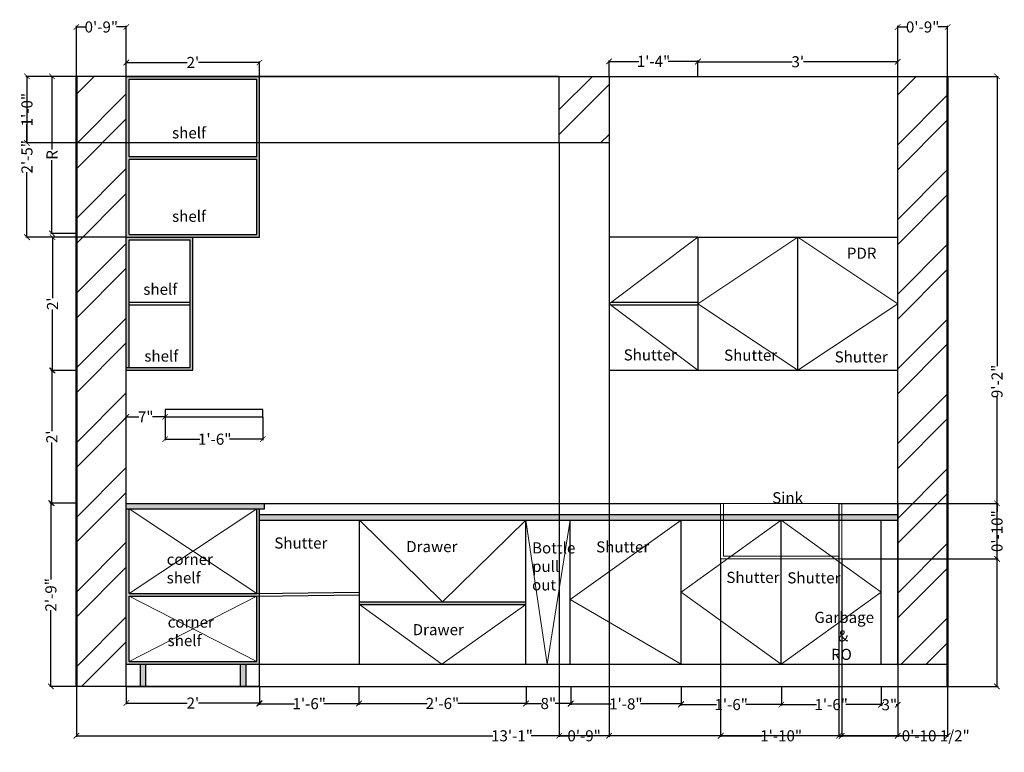
# Model space of a CAD drawing. Units: inches. Extents: x 3107 to 3291, y 1339 to 1621.
# Tile 1 of 3: x 3109 to 3286, y 1339 to 1471. Entities that reach past the tile are written whole.
import ezdxf

# ---------------------------------------------------------------- set-up
doc = ezdxf.new("R2010")
doc.units = ezdxf.units.IN
for name, color, linetype, lineweight in [('A-ANNO-DIMS', 2, 'Continuous', 18), ('A-ANNO-TEXT', 7, 'Continuous', 18), ('A-ELEV', 7, 'Continuous', 25), ('A-ELEV-OPEN', 165, 'Continuous', 13), ('A-ELEV-PATT', 8, 'Continuous', 13), ('A-FLOR-FIXT', 5, 'Continuous', 18), ('A-WALL', 7, 'Continuous', 50), ('A-WALL-PATT', 8, 'Continuous', 13)]:
    doc.layers.add(name, color=color, linetype=linetype, lineweight=lineweight)
doc.styles.get("Standard").update_dxf_attribs({"font": 'arial.ttf', "height": 2})
doc.dimstyles.get("Standard").update_dxf_attribs({"dimtxt": 2, "dimasz": 1, "dimexe": 0.18, "dimexo": 0.0625, "dimgap": 0.09, "dimtad": 0, "dimdec": 0, "dimzin": 0, "dimdsep": 46, "dimlunit": 3, "dimtxsty": 'Standard', "dimblk": 'ARCHTICK', "dimcen": 0.09, "dimadec": 0, "dimazin": 0, "dimtfac": 1, "dimtdec": 0, "dimtofl": 0, "dimtmove": 0, "dimatfit": 3, "dimfxl": 1, "dimtolj": 1, "dimtzin": 0, "dimarcsym": 0})

# ---------------------------------------------------------------- blocks, each defined once
blk = doc.blocks.new('_ArchTick')
at = {"color": 0, "linetype": 'ByBlock', "const_width": 0.15}
blk.add_lwpolyline([(-0.5, -0.5), (0.5, 0.5)], dxfattribs=at)
blk = doc.blocks.new('*D1')
at = {"layer": 'A-ANNO-DIMS', "color": 0, "lineweight": -2, "transparency": 16777216}
for p, q in [((3231.26, 1461.17), (3231.26, 1463.91)), ((3267.26, 1461.17), (3267.26, 1463.91)), ((3231.26, 1463.73), (3248.25, 1463.73)), ((3267.26, 1463.73), (3250.27, 1463.73))]:
    blk.add_line(p, q, dxfattribs=at)
at = {"layer": 'Defpoints', "color": 0, "transparency": 16777216}
for p in [(3231.26, 1463.73), (3231.26, 1461.1), (3267.26, 1461.1)]:
    blk.add_point(p, dxfattribs=at)
at = {"layer": 'A-ANNO-DIMS', "color": 0, "lineweight": -2, "transparency": 16777216, "rotation": 180}
blk.add_blockref('_ArchTick', (3231.26, 1463.73), dxfattribs=at)
at = {"layer": 'A-ANNO-DIMS', "color": 0, "lineweight": -2, "transparency": 16777216}
blk.add_blockref('_ArchTick', (3267.26, 1463.73), dxfattribs=at)
at = {"layer": 'A-ANNO-DIMS', "color": 0, "transparency": 16777216, "insert": (3249.26, 1463.73), "char_height": 2, "attachment_point": 5}
blk.add_mtext("\\A1;3'", dxfattribs=at)
blk = doc.blocks.new('*D2')
at = {"layer": 'A-ANNO-DIMS', "color": 0, "lineweight": -2, "transparency": 16777216}
for p, q in [((3215.26, 1461.17), (3215.26, 1463.98)), ((3215.26, 1463.8), (3220.61, 1463.8)), ((3231.26, 1463.8), (3225.92, 1463.8)), ((3231.26, 1461.17), (3231.26, 1463.98))]:
    blk.add_line(p, q, dxfattribs=at)
at = {"layer": 'Defpoints', "color": 0, "transparency": 16777216}
for p in [(3215.26, 1463.8), (3215.26, 1461.1), (3231.26, 1461.1)]:
    blk.add_point(p, dxfattribs=at)
at = {"layer": 'A-ANNO-DIMS', "color": 0, "lineweight": -2, "transparency": 16777216, "rotation": 180}
blk.add_blockref('_ArchTick', (3215.26, 1463.8), dxfattribs=at)
at = {"layer": 'A-ANNO-DIMS', "color": 0, "lineweight": -2, "transparency": 16777216}
blk.add_blockref('_ArchTick', (3231.26, 1463.8), dxfattribs=at)
at = {"layer": 'A-ANNO-DIMS', "color": 0, "transparency": 16777216, "insert": (3223.26, 1463.8), "char_height": 2, "attachment_point": 5}
blk.add_mtext('\\A1;1\'-4"', dxfattribs=at)
blk = doc.blocks.new('*D3')
at = {"layer": 'A-ANNO-DIMS', "color": 0, "lineweight": -2, "transparency": 16777216}
for p, q in [((3128.26, 1399.77), (3128.26, 1399.88)), ((3135.26, 1399.77), (3135.26, 1399.88)), ((3128.26, 1399.7), (3130.53, 1399.7)), ((3135.26, 1399.7), (3132.99, 1399.7))]:
    blk.add_line(p, q, dxfattribs=at)
at = {"layer": 'Defpoints', "color": 0, "transparency": 16777216}
for p in [(3128.26, 1399.7), (3128.26, 1399.7), (3135.26, 1399.7)]:
    blk.add_point(p, dxfattribs=at)
at = {"layer": 'A-ANNO-DIMS', "color": 0, "lineweight": -2, "transparency": 16777216, "rotation": 180}
blk.add_blockref('_ArchTick', (3128.26, 1399.7), dxfattribs=at)
at = {"layer": 'A-ANNO-DIMS', "color": 0, "lineweight": -2, "transparency": 16777216}
blk.add_blockref('_ArchTick', (3135.26, 1399.7), dxfattribs=at)
at = {"layer": 'A-ANNO-DIMS', "color": 0, "transparency": 16777216, "insert": (3131.76, 1399.7), "char_height": 2, "attachment_point": 5}
blk.add_mtext('\\A1;7"', dxfattribs=at)
blk = doc.blocks.new('*D4')
at = {"layer": 'A-ANNO-DIMS', "color": 0, "lineweight": -2, "transparency": 16777216}
for p, q in [((3135.26, 1399.64), (3135.26, 1395.5)), ((3152.87, 1399.64), (3152.87, 1395.5)), ((3135.26, 1395.68), (3141.53, 1395.68)), ((3152.87, 1395.68), (3146.84, 1395.68))]:
    blk.add_line(p, q, dxfattribs=at)
at = {"layer": 'Defpoints', "color": 0, "transparency": 16777216}
for p in [(3135.26, 1399.7), (3152.87, 1399.7), (3152.87, 1395.68)]:
    blk.add_point(p, dxfattribs=at)
at = {"layer": 'A-ANNO-DIMS', "color": 0, "lineweight": -2, "transparency": 16777216, "rotation": 180}
blk.add_blockref('_ArchTick', (3135.26, 1395.68), dxfattribs=at)
at = {"layer": 'A-ANNO-DIMS', "color": 0, "lineweight": -2, "transparency": 16777216}
blk.add_blockref('_ArchTick', (3152.87, 1395.68), dxfattribs=at)
at = {"layer": 'A-ANNO-DIMS', "color": 0, "transparency": 16777216, "insert": (3144.19, 1395.68), "char_height": 2, "attachment_point": 5}
blk.add_mtext('\\A1;1\'-6"', dxfattribs=at)
blk = doc.blocks.new('*D5')
at = {"layer": 'A-ANNO-DIMS', "color": 0, "lineweight": -2, "transparency": 16777216}
for p, q in [((3128.26, 1461.17), (3128.26, 1463.78)), ((3152.26, 1461.17), (3152.26, 1463.78)), ((3128.26, 1463.6), (3139.24, 1463.6)), ((3152.26, 1463.6), (3141.29, 1463.6))]:
    blk.add_line(p, q, dxfattribs=at)
at = {"layer": 'Defpoints', "color": 0, "transparency": 16777216}
for p in [(3152.26, 1463.6), (3128.26, 1461.1), (3152.26, 1461.1)]:
    blk.add_point(p, dxfattribs=at)
at = {"layer": 'A-ANNO-DIMS', "color": 0, "lineweight": -2, "transparency": 16777216, "rotation": 180}
blk.add_blockref('_ArchTick', (3128.26, 1463.6), dxfattribs=at)
at = {"layer": 'A-ANNO-DIMS', "color": 0, "lineweight": -2, "transparency": 16777216}
blk.add_blockref('_ArchTick', (3152.26, 1463.6), dxfattribs=at)
at = {"layer": 'A-ANNO-DIMS', "color": 0, "transparency": 16777216, "insert": (3140.26, 1463.6), "char_height": 2, "attachment_point": 5}
blk.add_mtext("\\A1;2'", dxfattribs=at)
blk = doc.blocks.new('*D8')
at = {"layer": 'A-ANNO-DIMS', "color": 0, "lineweight": -2, "transparency": 16777216}
for p, q in [((3119.2, 1461.1), (3114.69, 1461.1)), ((3114.87, 1461.1), (3114.87, 1447.9)), ((3114.87, 1432.76), (3114.87, 1445.96)), ((3119.2, 1432.76), (3114.69, 1432.76))]:
    blk.add_line(p, q, dxfattribs=at)
at = {"layer": 'Defpoints', "color": 0, "transparency": 16777216}
for p in [(3119.26, 1461.1), (3114.87, 1432.76), (3119.26, 1432.76)]:
    blk.add_point(p, dxfattribs=at)
at = {"layer": 'A-ANNO-DIMS', "color": 0, "lineweight": -2, "transparency": 16777216}
for p, rotation in [((3114.87, 1461.1), 90), ((3114.87, 1432.76), 270)]:
    blk.add_blockref('_ArchTick', p, dxfattribs=dict(at, rotation=rotation))
at = {"layer": 'A-ANNO-DIMS', "color": 0, "transparency": 16777216, "insert": (3114.87, 1446.93), "char_height": 2, "attachment_point": 5, "rotation": 90}
blk.add_mtext('\\A1;R', dxfattribs=at)
blk = doc.blocks.new('*D9')
at = {"layer": 'A-ANNO-DIMS', "color": 0, "lineweight": -2, "transparency": 16777216}
for p, q in [((3119.2, 1432.1), (3114.79, 1432.1)), ((3114.97, 1432.1), (3114.97, 1421.12)), ((3114.97, 1408.08), (3114.97, 1419.06)), ((3119.2, 1408.08), (3114.79, 1408.08))]:
    blk.add_line(p, q, dxfattribs=at)
at = {"layer": 'Defpoints', "color": 0, "transparency": 16777216}
for p in [(3119.26, 1432.1), (3114.97, 1408.08), (3119.26, 1408.08)]:
    blk.add_point(p, dxfattribs=at)
at = {"layer": 'A-ANNO-DIMS', "color": 0, "lineweight": -2, "transparency": 16777216}
for p, rotation in [((3114.97, 1432.1), 90), ((3114.97, 1408.08), 270)]:
    blk.add_blockref('_ArchTick', p, dxfattribs=dict(at, rotation=rotation))
at = {"layer": 'A-ANNO-DIMS', "color": 0, "transparency": 16777216, "insert": (3114.97, 1420.09), "char_height": 2, "attachment_point": 5, "rotation": 90}
blk.add_mtext("\\A1;2'", dxfattribs=at)
blk = doc.blocks.new('*D10')
at = {"layer": 'A-ANNO-DIMS', "color": 0, "lineweight": -2, "transparency": 16777216}
for p, q in [((3119.2, 1408.08), (3114.66, 1408.08)), ((3114.84, 1408.08), (3114.84, 1397.14)), ((3114.84, 1384.14), (3114.84, 1395.08)), ((3119.2, 1384.14), (3114.66, 1384.14))]:
    blk.add_line(p, q, dxfattribs=at)
at = {"layer": 'Defpoints', "color": 0, "transparency": 16777216}
for p in [(3119.26, 1408.08), (3114.84, 1384.14), (3119.26, 1384.14)]:
    blk.add_point(p, dxfattribs=at)
at = {"layer": 'A-ANNO-DIMS', "color": 0, "lineweight": -2, "transparency": 16777216}
for p, rotation in [((3114.84, 1408.08), 90), ((3114.84, 1384.14), 270)]:
    blk.add_blockref('_ArchTick', p, dxfattribs=dict(at, rotation=rotation))
at = {"layer": 'A-ANNO-DIMS', "color": 0, "transparency": 16777216, "insert": (3114.84, 1396.11), "char_height": 2, "attachment_point": 5, "rotation": 90}
blk.add_mtext("\\A1;2'", dxfattribs=at)
blk = doc.blocks.new('*D11')
at = {"layer": 'A-ANNO-DIMS', "color": 0, "lineweight": -2, "transparency": 16777216}
for p, q in [((3119.2, 1384.14), (3114.49, 1384.14)), ((3114.67, 1384.14), (3114.67, 1370.39)), ((3114.67, 1351.1), (3114.67, 1364.86)), ((3119.2, 1351.1), (3114.49, 1351.1))]:
    blk.add_line(p, q, dxfattribs=at)
at = {"layer": 'Defpoints', "color": 0, "transparency": 16777216}
for p in [(3119.26, 1384.14), (3114.67, 1351.1), (3119.26, 1351.1)]:
    blk.add_point(p, dxfattribs=at)
at = {"layer": 'A-ANNO-DIMS', "color": 0, "lineweight": -2, "transparency": 16777216}
for p, rotation in [((3114.67, 1384.14), 90), ((3114.67, 1351.1), 270)]:
    blk.add_blockref('_ArchTick', p, dxfattribs=dict(at, rotation=rotation))
at = {"layer": 'A-ANNO-DIMS', "color": 0, "transparency": 16777216, "insert": (3114.67, 1367.62), "char_height": 2, "attachment_point": 5, "rotation": 90}
blk.add_mtext('\\A1;2\'-9"', dxfattribs=at)
blk = doc.blocks.new('*D12')
at = {"layer": 'A-ANNO-DIMS', "color": 0, "lineweight": -2, "transparency": 16777216}
for p, q in [((3128.26, 1351.04), (3128.26, 1347.92)), ((3152.26, 1351.04), (3152.26, 1347.92)), ((3128.26, 1348.1), (3139.24, 1348.1)), ((3152.26, 1348.1), (3141.29, 1348.1))]:
    blk.add_line(p, q, dxfattribs=at)
at = {"layer": 'Defpoints', "color": 0, "transparency": 16777216}
for p in [(3128.26, 1351.1), (3152.26, 1351.1), (3152.26, 1348.1)]:
    blk.add_point(p, dxfattribs=at)
at = {"layer": 'A-ANNO-DIMS', "color": 0, "lineweight": -2, "transparency": 16777216, "rotation": 180}
blk.add_blockref('_ArchTick', (3128.26, 1348.1), dxfattribs=at)
at = {"layer": 'A-ANNO-DIMS', "color": 0, "lineweight": -2, "transparency": 16777216}
blk.add_blockref('_ArchTick', (3152.26, 1348.1), dxfattribs=at)
at = {"layer": 'A-ANNO-DIMS', "color": 0, "transparency": 16777216, "insert": (3140.26, 1348.1), "char_height": 2, "attachment_point": 5}
blk.add_mtext("\\A1;2'", dxfattribs=at)
blk = doc.blocks.new('*D13')
at = {"layer": 'A-ANNO-DIMS', "color": 0, "lineweight": -2, "transparency": 16777216}
for p, q in [((3152.26, 1351.04), (3152.26, 1347.81)), ((3170.18, 1351.04), (3170.18, 1347.81)), ((3152.26, 1347.99), (3158.57, 1347.99)), ((3170.18, 1347.99), (3163.87, 1347.99))]:
    blk.add_line(p, q, dxfattribs=at)
at = {"layer": 'Defpoints', "color": 0, "transparency": 16777216}
for p in [(3152.26, 1351.1), (3170.18, 1351.1), (3170.18, 1347.99)]:
    blk.add_point(p, dxfattribs=at)
at = {"layer": 'A-ANNO-DIMS', "color": 0, "lineweight": -2, "transparency": 16777216, "rotation": 180}
blk.add_blockref('_ArchTick', (3152.26, 1347.99), dxfattribs=at)
at = {"layer": 'A-ANNO-DIMS', "color": 0, "lineweight": -2, "transparency": 16777216}
blk.add_blockref('_ArchTick', (3170.18, 1347.99), dxfattribs=at)
at = {"layer": 'A-ANNO-DIMS', "color": 0, "transparency": 16777216, "insert": (3161.22, 1347.99), "char_height": 2, "attachment_point": 5}
blk.add_mtext('\\A1;1\'-6"', dxfattribs=at)
blk = doc.blocks.new('*D14')
at = {"layer": 'A-ANNO-DIMS', "color": 0, "lineweight": -2, "transparency": 16777216}
for p, q in [((3170.18, 1351.04), (3170.18, 1347.85)), ((3200.29, 1351.04), (3200.29, 1347.85)), ((3170.18, 1348.03), (3182.47, 1348.03)), ((3200.29, 1348.03), (3188, 1348.03))]:
    blk.add_line(p, q, dxfattribs=at)
at = {"layer": 'Defpoints', "color": 0, "transparency": 16777216}
for p in [(3170.18, 1351.1), (3200.29, 1351.1), (3200.29, 1348.03)]:
    blk.add_point(p, dxfattribs=at)
at = {"layer": 'A-ANNO-DIMS', "color": 0, "lineweight": -2, "transparency": 16777216, "rotation": 180}
blk.add_blockref('_ArchTick', (3170.18, 1348.03), dxfattribs=at)
at = {"layer": 'A-ANNO-DIMS', "color": 0, "lineweight": -2, "transparency": 16777216}
blk.add_blockref('_ArchTick', (3200.29, 1348.03), dxfattribs=at)
at = {"layer": 'A-ANNO-DIMS', "color": 0, "transparency": 16777216, "insert": (3185.23, 1348.03), "char_height": 2, "attachment_point": 5}
blk.add_mtext('\\A1;2\'-6"', dxfattribs=at)
blk = doc.blocks.new('*D15')
at = {"layer": 'A-ANNO-DIMS', "color": 0, "lineweight": -2, "transparency": 16777216}
for p, q in [((3200.29, 1351.04), (3200.29, 1347.84)), ((3208.34, 1351.04), (3208.34, 1347.84)), ((3200.29, 1348.02), (3203.07, 1348.02)), ((3208.34, 1348.02), (3205.55, 1348.02))]:
    blk.add_line(p, q, dxfattribs=at)
at = {"layer": 'Defpoints', "color": 0, "transparency": 16777216}
for p in [(3200.29, 1351.1), (3208.34, 1351.1), (3208.34, 1348.02)]:
    blk.add_point(p, dxfattribs=at)
at = {"layer": 'A-ANNO-DIMS', "color": 0, "lineweight": -2, "transparency": 16777216, "rotation": 180}
blk.add_blockref('_ArchTick', (3200.29, 1348.02), dxfattribs=at)
at = {"layer": 'A-ANNO-DIMS', "color": 0, "lineweight": -2, "transparency": 16777216}
blk.add_blockref('_ArchTick', (3208.34, 1348.02), dxfattribs=at)
at = {"layer": 'A-ANNO-DIMS', "color": 0, "transparency": 16777216, "insert": (3204.31, 1348.02), "char_height": 2, "attachment_point": 5}
blk.add_mtext('\\A1;8"', dxfattribs=at)
blk = doc.blocks.new('*D16')
at = {"layer": 'A-ANNO-DIMS', "color": 0, "lineweight": -2, "transparency": 16777216}
for p, q in [((3208.34, 1351.04), (3208.34, 1347.77)), ((3228.23, 1351.04), (3228.23, 1347.77)), ((3208.34, 1347.95), (3215.63, 1347.95)), ((3228.23, 1347.95), (3220.94, 1347.95))]:
    blk.add_line(p, q, dxfattribs=at)
at = {"layer": 'Defpoints', "color": 0, "transparency": 16777216}
for p in [(3208.34, 1351.1), (3228.23, 1351.1), (3228.23, 1347.95)]:
    blk.add_point(p, dxfattribs=at)
at = {"layer": 'A-ANNO-DIMS', "color": 0, "lineweight": -2, "transparency": 16777216, "rotation": 180}
blk.add_blockref('_ArchTick', (3208.34, 1347.95), dxfattribs=at)
at = {"layer": 'A-ANNO-DIMS', "color": 0, "lineweight": -2, "transparency": 16777216}
blk.add_blockref('_ArchTick', (3228.23, 1347.95), dxfattribs=at)
at = {"layer": 'A-ANNO-DIMS', "color": 0, "transparency": 16777216, "insert": (3218.28, 1347.95), "char_height": 2, "attachment_point": 5}
blk.add_mtext('\\A1;1\'-8"', dxfattribs=at)
blk = doc.blocks.new('*D17')
at = {"layer": 'A-ANNO-DIMS', "color": 0, "lineweight": -2, "transparency": 16777216}
for p, q in [((3228.23, 1351.04), (3228.23, 1347.65)), ((3246.3, 1351.04), (3246.3, 1347.65)), ((3228.23, 1347.83), (3234.61, 1347.83)), ((3246.3, 1347.83), (3239.92, 1347.83))]:
    blk.add_line(p, q, dxfattribs=at)
at = {"layer": 'Defpoints', "color": 0, "transparency": 16777216}
for p in [(3228.23, 1351.1), (3246.3, 1351.1), (3246.3, 1347.83)]:
    blk.add_point(p, dxfattribs=at)
at = {"layer": 'A-ANNO-DIMS', "color": 0, "lineweight": -2, "transparency": 16777216, "rotation": 180}
blk.add_blockref('_ArchTick', (3228.23, 1347.83), dxfattribs=at)
at = {"layer": 'A-ANNO-DIMS', "color": 0, "lineweight": -2, "transparency": 16777216}
blk.add_blockref('_ArchTick', (3246.3, 1347.83), dxfattribs=at)
at = {"layer": 'A-ANNO-DIMS', "color": 0, "transparency": 16777216, "insert": (3237.26, 1347.83), "char_height": 2, "attachment_point": 5}
blk.add_mtext('\\A1;1\'-6"', dxfattribs=at)
blk = doc.blocks.new('*D18')
at = {"layer": 'A-ANNO-DIMS', "color": 0, "lineweight": -2, "transparency": 16777216}
for p, q in [((3246.3, 1351.04), (3246.3, 1347.65)), ((3264.26, 1351.04), (3264.26, 1347.65)), ((3246.3, 1347.83), (3252.63, 1347.83)), ((3264.26, 1347.83), (3257.93, 1347.83))]:
    blk.add_line(p, q, dxfattribs=at)
at = {"layer": 'Defpoints', "color": 0, "transparency": 16777216}
for p in [(3246.3, 1351.1), (3264.26, 1351.1), (3264.26, 1347.83)]:
    blk.add_point(p, dxfattribs=at)
at = {"layer": 'A-ANNO-DIMS', "color": 0, "lineweight": -2, "transparency": 16777216, "rotation": 180}
blk.add_blockref('_ArchTick', (3246.3, 1347.83), dxfattribs=at)
at = {"layer": 'A-ANNO-DIMS', "color": 0, "lineweight": -2, "transparency": 16777216}
blk.add_blockref('_ArchTick', (3264.26, 1347.83), dxfattribs=at)
at = {"layer": 'A-ANNO-DIMS', "color": 0, "transparency": 16777216, "insert": (3255.28, 1347.83), "char_height": 2, "attachment_point": 5}
blk.add_mtext('\\A1;1\'-6"', dxfattribs=at)
blk = doc.blocks.new('*D19')
at = {"layer": 'A-ANNO-DIMS', "color": 0, "lineweight": -2, "transparency": 16777216}
for p, q in [((3264.26, 1351.04), (3264.26, 1347.62)), ((3267.26, 1351.04), (3267.26, 1347.62)), ((3264.26, 1347.8), (3264.52, 1347.8)), ((3267.26, 1347.8), (3267, 1347.8))]:
    blk.add_line(p, q, dxfattribs=at)
at = {"layer": 'Defpoints', "color": 0, "transparency": 16777216}
for p in [(3264.26, 1351.1), (3267.26, 1351.1), (3267.26, 1347.8)]:
    blk.add_point(p, dxfattribs=at)
at = {"layer": 'A-ANNO-DIMS', "color": 0, "lineweight": -2, "transparency": 16777216, "rotation": 180}
blk.add_blockref('_ArchTick', (3264.26, 1347.8), dxfattribs=at)
at = {"layer": 'A-ANNO-DIMS', "color": 0, "lineweight": -2, "transparency": 16777216}
blk.add_blockref('_ArchTick', (3267.26, 1347.8), dxfattribs=at)
at = {"layer": 'A-ANNO-DIMS', "color": 0, "transparency": 16777216, "insert": (3265.76, 1347.8), "char_height": 2, "attachment_point": 5}
blk.add_mtext('\\A1;3"', dxfattribs=at)
blk = doc.blocks.new('*D68')
at = {"layer": 'A-ANNO-DIMS', "color": 0, "lineweight": -2, "transparency": 16777216}
for p, q in [((3119.26, 1351.04), (3119.26, 1342.02)), ((3276.26, 1351.04), (3276.26, 1342.02)), ((3119.26, 1342.2), (3194.33, 1342.2)), ((3276.26, 1342.2), (3201.19, 1342.2))]:
    blk.add_line(p, q, dxfattribs=at)
at = {"layer": 'Defpoints', "color": 0, "transparency": 16777216}
for p in [(3119.26, 1351.1), (3276.26, 1351.1), (3276.26, 1342.2)]:
    blk.add_point(p, dxfattribs=at)
at = {"layer": 'A-ANNO-DIMS', "color": 0, "lineweight": -2, "transparency": 16777216, "rotation": 180}
blk.add_blockref('_ArchTick', (3119.26, 1342.2), dxfattribs=at)
at = {"layer": 'A-ANNO-DIMS', "color": 0, "lineweight": -2, "transparency": 16777216}
blk.add_blockref('_ArchTick', (3276.26, 1342.2), dxfattribs=at)
at = {"layer": 'A-ANNO-DIMS', "color": 0, "transparency": 16777216, "insert": (3197.76, 1342.2), "char_height": 2, "attachment_point": 5}
blk.add_mtext('\\A1;13\'-1"', dxfattribs=at)
blk = doc.blocks.new('*D69')
at = {"layer": 'A-ANNO-DIMS', "color": 0, "lineweight": -2, "transparency": 16777216}
for p, q in [((3276.32, 1461.1), (3285.34, 1461.1)), ((3285.16, 1461.1), (3285.16, 1408.85)), ((3285.16, 1351.1), (3285.16, 1403.36)), ((3276.32, 1351.1), (3285.34, 1351.1))]:
    blk.add_line(p, q, dxfattribs=at)
at = {"layer": 'Defpoints', "color": 0, "transparency": 16777216}
for p in [(3276.26, 1461.1), (3285.16, 1461.1), (3276.26, 1351.1)]:
    blk.add_point(p, dxfattribs=at)
at = {"layer": 'A-ANNO-DIMS', "color": 0, "lineweight": -2, "transparency": 16777216}
for p, rotation in [((3285.16, 1461.1), 90), ((3285.16, 1351.1), 270)]:
    blk.add_blockref('_ArchTick', p, dxfattribs=dict(at, rotation=rotation))
at = {"layer": 'A-ANNO-DIMS', "color": 0, "transparency": 16777216, "insert": (3285.16, 1406.1), "char_height": 2, "attachment_point": 5, "rotation": 90}
blk.add_mtext('\\A1;9\'-2"', dxfattribs=at)
blk = doc.blocks.new('*D70')
at = {"layer": 'A-ANNO-DIMS', "color": 0, "lineweight": -2, "transparency": 16777216}
for p, q in [((3128.2, 1461.1), (3110.18, 1461.1)), ((3110.36, 1461.1), (3110.36, 1449.37)), ((3110.36, 1432.1), (3110.36, 1443.84)), ((3128.2, 1432.1), (3110.18, 1432.1))]:
    blk.add_line(p, q, dxfattribs=at)
at = {"layer": 'Defpoints', "color": 0, "transparency": 16777216}
for p in [(3110.36, 1461.1), (3128.26, 1461.1), (3128.26, 1432.1)]:
    blk.add_point(p, dxfattribs=at)
at = {"layer": 'A-ANNO-DIMS', "color": 0, "lineweight": -2, "transparency": 16777216}
for p, rotation in [((3110.36, 1461.1), 90), ((3110.36, 1432.1), 270)]:
    blk.add_blockref('_ArchTick', p, dxfattribs=dict(at, rotation=rotation))
at = {"layer": 'A-ANNO-DIMS', "color": 0, "transparency": 16777216, "insert": (3110.36, 1446.6), "char_height": 2, "attachment_point": 5, "rotation": 90}
blk.add_mtext('\\A1;2\'-5"', dxfattribs=at)
blk = doc.blocks.new('*D71')
at = {"layer": 'A-ANNO-DIMS', "color": 0, "lineweight": -2, "transparency": 16777216}
for p, q in [((3119.26, 1461.17), (3119.26, 1470.18)), ((3119.26, 1470), (3121.01, 1470)), ((3128.26, 1470), (3126.51, 1470)), ((3128.26, 1461.17), (3128.26, 1470.18))]:
    blk.add_line(p, q, dxfattribs=at)
at = {"layer": 'Defpoints', "color": 0, "transparency": 16777216}
for p in [(3128.26, 1470), (3119.26, 1461.1), (3128.26, 1461.1)]:
    blk.add_point(p, dxfattribs=at)
at = {"layer": 'A-ANNO-DIMS', "color": 0, "lineweight": -2, "transparency": 16777216, "rotation": 180}
blk.add_blockref('_ArchTick', (3119.26, 1470), dxfattribs=at)
at = {"layer": 'A-ANNO-DIMS', "color": 0, "lineweight": -2, "transparency": 16777216}
blk.add_blockref('_ArchTick', (3128.26, 1470), dxfattribs=at)
at = {"layer": 'A-ANNO-DIMS', "color": 0, "transparency": 16777216, "insert": (3123.76, 1470), "char_height": 2, "attachment_point": 5}
blk.add_mtext('\\A1;0\'-9"', dxfattribs=at)
blk = doc.blocks.new('*D72')
at = {"layer": 'A-ANNO-DIMS', "color": 0, "lineweight": -2, "transparency": 16777216}
for p, q in [((3267.26, 1461.17), (3267.26, 1470.18)), ((3267.26, 1470), (3269.01, 1470)), ((3276.26, 1470), (3274.51, 1470)), ((3276.26, 1461.17), (3276.26, 1470.18))]:
    blk.add_line(p, q, dxfattribs=at)
at = {"layer": 'Defpoints', "color": 0, "transparency": 16777216}
for p in [(3276.26, 1470), (3267.26, 1461.1), (3276.26, 1461.1)]:
    blk.add_point(p, dxfattribs=at)
at = {"layer": 'A-ANNO-DIMS', "color": 0, "lineweight": -2, "transparency": 16777216, "rotation": 180}
blk.add_blockref('_ArchTick', (3267.26, 1470), dxfattribs=at)
at = {"layer": 'A-ANNO-DIMS', "color": 0, "lineweight": -2, "transparency": 16777216}
blk.add_blockref('_ArchTick', (3276.26, 1470), dxfattribs=at)
at = {"layer": 'A-ANNO-DIMS', "color": 0, "transparency": 16777216, "insert": (3271.76, 1470), "char_height": 2, "attachment_point": 5}
blk.add_mtext('\\A1;0\'-9"', dxfattribs=at)
blk = doc.blocks.new('*D73')
at = {"layer": 'A-ANNO-DIMS', "color": 0, "lineweight": -2, "transparency": 16777216}
for p, q in [((3206.2, 1461.1), (3110.18, 1461.1)), ((3110.36, 1461.1), (3110.36, 1457.76)), ((3110.36, 1449.1), (3110.36, 1452.45)), ((3206.2, 1449.1), (3110.18, 1449.1))]:
    blk.add_line(p, q, dxfattribs=at)
at = {"layer": 'Defpoints', "color": 0, "transparency": 16777216}
for p in [(3110.36, 1461.1), (3206.26, 1461.1), (3206.26, 1449.1)]:
    blk.add_point(p, dxfattribs=at)
at = {"layer": 'A-ANNO-DIMS', "color": 0, "lineweight": -2, "transparency": 16777216}
for p, rotation in [((3110.36, 1461.1), 90), ((3110.36, 1449.1), 270)]:
    blk.add_blockref('_ArchTick', p, dxfattribs=dict(at, rotation=rotation))
at = {"layer": 'A-ANNO-DIMS', "color": 0, "transparency": 16777216, "insert": (3110.36, 1455.1), "char_height": 2, "attachment_point": 5, "rotation": 90}
blk.add_mtext('\\A1;1\'-0"', dxfattribs=at)
blk = doc.blocks.new('*D74')
at = {"layer": 'A-ANNO-DIMS', "color": 0, "lineweight": -2, "transparency": 16777216}
for p, q in [((3206.26, 1449.04), (3206.26, 1342.02)), ((3215.26, 1449.04), (3215.26, 1342.02)), ((3206.26, 1342.2), (3208.01, 1342.2)), ((3215.26, 1342.2), (3213.51, 1342.2))]:
    blk.add_line(p, q, dxfattribs=at)
at = {"layer": 'Defpoints', "color": 0, "transparency": 16777216}
for p in [(3206.26, 1449.1), (3215.26, 1449.1), (3215.26, 1342.2)]:
    blk.add_point(p, dxfattribs=at)
at = {"layer": 'A-ANNO-DIMS', "color": 0, "lineweight": -2, "transparency": 16777216, "rotation": 180}
blk.add_blockref('_ArchTick', (3206.26, 1342.2), dxfattribs=at)
at = {"layer": 'A-ANNO-DIMS', "color": 0, "lineweight": -2, "transparency": 16777216}
blk.add_blockref('_ArchTick', (3215.26, 1342.2), dxfattribs=at)
at = {"layer": 'A-ANNO-DIMS', "color": 0, "transparency": 16777216, "insert": (3210.76, 1342.2), "char_height": 2, "attachment_point": 5}
blk.add_mtext('\\A1;0\'-9"', dxfattribs=at)
blk = doc.blocks.new('*D75')
at = {"layer": 'A-ANNO-DIMS', "color": 0, "lineweight": -2, "transparency": 16777216}
for p, q in [((3235.36, 1374.04), (3235.36, 1342.02)), ((3257.17, 1374.04), (3257.17, 1342.02)), ((3235.36, 1342.2), (3242.83, 1342.2)), ((3257.17, 1342.2), (3249.69, 1342.2))]:
    blk.add_line(p, q, dxfattribs=at)
at = {"layer": 'Defpoints', "color": 0, "transparency": 16777216}
for p in [(3235.36, 1374.1), (3257.17, 1374.1), (3257.17, 1342.2)]:
    blk.add_point(p, dxfattribs=at)
at = {"layer": 'A-ANNO-DIMS', "color": 0, "lineweight": -2, "transparency": 16777216, "rotation": 180}
blk.add_blockref('_ArchTick', (3235.36, 1342.2), dxfattribs=at)
at = {"layer": 'A-ANNO-DIMS', "color": 0, "lineweight": -2, "transparency": 16777216}
blk.add_blockref('_ArchTick', (3257.17, 1342.2), dxfattribs=at)
at = {"layer": 'A-ANNO-DIMS', "color": 0, "transparency": 16777216, "insert": (3246.26, 1342.2), "char_height": 2, "attachment_point": 5}
blk.add_mtext('\\A1;1\'-10"', dxfattribs=at)
blk = doc.blocks.new('*D76')
at = {"layer": 'A-ANNO-DIMS', "color": 0, "lineweight": -2, "transparency": 16777216}
for p, q in [((3256.73, 1384.1), (3285.34, 1384.1)), ((3285.16, 1384.1), (3285.16, 1382.63)), ((3285.16, 1374.1), (3285.16, 1375.58)), ((3257.23, 1374.1), (3285.34, 1374.1))]:
    blk.add_line(p, q, dxfattribs=at)
at = {"layer": 'Defpoints', "color": 0, "transparency": 16777216}
for p in [(3256.67, 1384.1), (3285.16, 1384.1), (3257.17, 1374.1)]:
    blk.add_point(p, dxfattribs=at)
at = {"layer": 'A-ANNO-DIMS', "color": 0, "lineweight": -2, "transparency": 16777216}
for p, rotation in [((3285.16, 1384.1), 90), ((3285.16, 1374.1), 270)]:
    blk.add_blockref('_ArchTick', p, dxfattribs=dict(at, rotation=rotation))
at = {"layer": 'A-ANNO-DIMS', "color": 0, "transparency": 16777216, "insert": (3285.16, 1379.1), "char_height": 2, "attachment_point": 5, "rotation": 90}
blk.add_mtext('\\A1;0\'-10"', dxfattribs=at)
blk = doc.blocks.new('*D77')
at = {"layer": 'A-ANNO-DIMS', "color": 0, "lineweight": -2, "transparency": 16777216}
for p, q in [((3256.67, 1384.04), (3256.67, 1342.02)), ((3267.26, 1384.04), (3267.26, 1342.02)), ((3256.67, 1342.2), (3267.26, 1342.2)), ((3267.26, 1342.2), (3268.26, 1342.2))]:
    blk.add_line(p, q, dxfattribs=at)
at = {"layer": 'Defpoints', "color": 0, "transparency": 16777216}
for p in [(3256.67, 1384.1), (3267.26, 1384.1), (3267.26, 1342.2)]:
    blk.add_point(p, dxfattribs=at)
at = {"layer": 'A-ANNO-DIMS', "color": 0, "lineweight": -2, "transparency": 16777216, "rotation": 180}
blk.add_blockref('_ArchTick', (3256.67, 1342.2), dxfattribs=at)
at = {"layer": 'A-ANNO-DIMS', "color": 0, "lineweight": -2, "transparency": 16777216}
blk.add_blockref('_ArchTick', (3267.26, 1342.2), dxfattribs=at)
at = {"layer": 'A-ANNO-DIMS', "color": 0, "transparency": 16777216, "insert": (3274.12, 1342.2), "char_height": 2, "attachment_point": 5}
blk.add_mtext('\\A1;0\'-10 1/2"', dxfattribs=at)

msp = doc.modelspace()

# ---------------------------------------------------------------- hatches: boundary and pattern name
at = {"layer": 'A-ELEV-PATT'}
h = msp.add_hatch(color=256, dxfattribs=at)
h.dxf.hatch_style = 1
h.paths.add_polyline_path([(3152.26, 1461.1), (3128.26, 1461.1), (3128.26, 1432.1), (3152.26, 1432.1)])
h.paths.add_polyline_path([(3151.76, 1446.6), (3128.76, 1446.6), (3128.76, 1460.6), (3151.76, 1460.6)], flags=16)
h.paths.add_polyline_path([(3151.76, 1446.1), (3151.76, 1432.6), (3128.76, 1432.6), (3128.76, 1446.1)], flags=16)
h.paths.add_polyline_path([(3140.26, 1432.1), (3128.26, 1432.1), (3128.26, 1408.6), (3128.76, 1408.6), (3128.76, 1431.6), (3139.76, 1431.6), (3139.76, 1408.6), (3128.26, 1408.6), (3128.26, 1408.1), (3140.26, 1408.1)])
h.paths.add_polyline_path([(3135.93, 1433.74), (3142.93, 1433.74), (3142.93, 1437.86), (3135.93, 1437.86)], flags=8)
h.paths.add_polyline_path([(3135.93, 1448.78), (3142.93, 1448.78), (3142.93, 1452.9), (3135.93, 1452.9)], flags=8)
h = msp.add_hatch(color=256, dxfattribs=at)
h.dxf.hatch_style = 1
h.paths.add_polyline_path([(3152.26, 1383.1), (3151.76, 1383.1), (3151.76, 1367.85), (3128.76, 1367.85), (3128.76, 1383.1), (3128.26, 1383.1), (3128.26, 1355.1), (3152.26, 1355.1)])
h.paths.add_polyline_path([(3151.76, 1355.6), (3128.76, 1355.6), (3128.76, 1367.35), (3151.76, 1367.35)], flags=16)
h.paths.add_polyline_path([(3149.8, 1355.1), (3148.8, 1355.1), (3148.8, 1351.1), (3149.8, 1351.1)])
h.paths.add_polyline_path([(3131.73, 1355.1), (3130.73, 1355.1), (3130.73, 1351.1), (3131.73, 1351.1)])
h.paths.add_polyline_path([(3153.14, 1384.1), (3128.26, 1384.1), (3128.26, 1383.1), (3128.76, 1383.1), (3153.14, 1383.1)])
h.paths.add_polyline_path([(3135.1, 1357.24), (3144.06, 1357.24), (3144.06, 1364.73), (3135.1, 1364.73)], flags=8)
h = msp.add_hatch(color=256, dxfattribs=at)
h.dxf.hatch_style = 1
h.paths.add_polyline_path([(3235.36, 1382.1), (3152.26, 1382.1), (3152.26, 1381.1), (3235.36, 1381.1)])
h = msp.add_hatch(color=256, dxfattribs=at)
h.dxf.hatch_style = 1
h.paths.add_polyline_path([(3256.67, 1382.1), (3235.86, 1382.1), (3235.86, 1381.1), (3256.67, 1381.1)])
h.paths.add_polyline_path([(3235.86, 1382.1), (3235.36, 1382.1), (3235.36, 1381.1), (3235.86, 1381.1)])
h.paths.add_polyline_path([(3257.17, 1382.1), (3256.67, 1382.1), (3256.67, 1381.1), (3257.17, 1381.1)])
h.paths.add_polyline_path([(3267.26, 1382.1), (3257.17, 1382.1), (3257.17, 1381.1), (3267.26, 1381.1)])
h = msp.add_hatch(color=256, dxfattribs=at)
h.dxf.hatch_style = 1
h.paths.add_polyline_path([(3200.26, 1366.35), (3170.26, 1366.35), (3170.26, 1365.85), (3200.26, 1365.85)])
at = {"layer": 'A-WALL-PATT'}
h = msp.add_hatch(dxfattribs=at)
h.set_pattern_fill('ANSI32', color=256)
h.paths.add_polyline_path([(3128.26, 1461.1), (3119.26, 1461.1), (3119.26, 1351.1), (3128.26, 1351.1)])
h.paths.add_polyline_path([(3276.26, 1461.1), (3267.26, 1461.1), (3267.26, 1432.1), (3267.26, 1408.1), (3267.26, 1355.1), (3276.26, 1355.1)])
h = msp.add_hatch(dxfattribs=at)
h.set_pattern_fill('ANSI32', color=256)
h.paths.add_polyline_path([(3215.26, 1461.1), (3206.26, 1461.1), (3206.26, 1449.1), (3215.26, 1449.1)])

# ---------------------------------------------------------------- linework, layer by layer
at = {"layer": 'A-ELEV'}
for p, q in [((3128.26, 1461.1), (3119.26, 1461.1)), ((3128.26, 1351.1), (3128.26, 1461.1)), ((3128.26, 1461.1), (3267.26, 1461.1)), ((3128.76, 1446.6), (3128.76, 1460.6)), ((3128.76, 1460.6), (3151.76, 1460.6)), ((3151.76, 1446.6), (3151.76, 1460.6)), ((3152.26, 1432.1), (3152.26, 1461.1)), ((3206.26, 1449.1), (3206.26, 1461.1)), ((3215.26, 1461.1), (3215.26, 1449.1)), ((3267.26, 1432.1), (3267.26, 1461.1)), ((3267.26, 1461.1), (3276.26, 1461.1)), ((3215.26, 1449.1), (3206.26, 1449.1)), ((3151.76, 1446.6), (3128.76, 1446.6)), ((3128.76, 1432.6), (3128.76, 1446.1)), ((3151.76, 1446.1), (3128.76, 1446.1)), ((3151.76, 1432.6), (3151.76, 1446.1)), ((3128.26, 1432.1), (3152.26, 1432.1)), ((3128.76, 1432.6), (3151.76, 1432.6)), ((3140.26, 1408.1), (3140.26, 1432.1)), ((3231.26, 1432.1), (3215.26, 1432.1)), ((3215.26, 1432.1), (3215.26, 1408.1)), ((3231.26, 1432.1), (3267.26, 1432.1)), ((3231.26, 1432.1), (3231.26, 1408.1)), ((3249.26, 1408.1), (3249.26, 1432.1)), ((3267.26, 1408.1), (3267.26, 1432.1)), ((3128.76, 1408.6), (3128.76, 1431.6)), ((3128.76, 1431.6), (3139.76, 1431.6)), ((3139.76, 1408.6), (3139.76, 1431.6)), ((3139.76, 1420.35), (3128.76, 1420.35)), ((3139.76, 1419.85), (3128.76, 1419.85)), ((3215.57, 1419.88), (3231.26, 1419.88)), ((3215.62, 1420.38), (3231.26, 1420.38)), ((3128.26, 1408.6), (3139.76, 1408.6)), ((3128.26, 1408.1), (3140.26, 1408.1)), ((3215.26, 1408.1), (3231.26, 1408.1)), ((3231.26, 1408.1), (3267.26, 1408.1)), ((3267.26, 1355.1), (3267.26, 1408.1)), ((3128.26, 1384.1), (3235.36, 1384.1)), ((3153.14, 1383.1), (3153.14, 1384.1)), ((3257.17, 1384.1), (3267.26, 1384.1)), ((3267.26, 1355.1), (3267.26, 1384.1)), ((3128.26, 1383.1), (3153.14, 1383.1)), ((3128.76, 1367.85), (3128.76, 1383.1)), ((3151.76, 1367.85), (3151.76, 1383.1)), ((3152.26, 1351.1), (3152.26, 1383.1)), ((3152.26, 1382.1), (3267.26, 1382.1)), ((3152.26, 1381.1), (3267.26, 1381.1)), ((3170.26, 1355.1), (3170.26, 1381.1)), ((3200.26, 1355.1), (3200.26, 1381.1)), ((3208.26, 1355.1), (3208.26, 1381.1)), ((3228.26, 1355.1), (3228.26, 1381.1)), ((3246.26, 1355.1), (3246.26, 1381.1)), ((3264.26, 1355.1), (3264.26, 1381.1)), ((3151.76, 1367.85), (3170.26, 1368.1)), ((3128.76, 1367.85), (3151.76, 1367.85)), ((3128.76, 1355.6), (3128.76, 1367.35)), ((3128.76, 1367.35), (3151.76, 1367.35)), ((3151.76, 1355.6), (3151.76, 1367.35)), ((3151.77, 1367.35), (3170.27, 1367.6)), ((3170.26, 1366.35), (3200.26, 1366.35)), ((3170.26, 1365.85), (3200.26, 1365.85)), ((3128.76, 1355.6), (3151.76, 1355.6)), ((3128.26, 1355.1), (3276.26, 1355.1)), ((3130.73, 1355.1), (3130.73, 1351.1)), ((3131.73, 1355.1), (3131.73, 1351.1)), ((3148.8, 1355.1), (3148.8, 1351.1)), ((3149.8, 1355.1), (3149.8, 1351.1)), ((3152.26, 1351.1), (3119.26, 1351.1)), ((3128.26, 1351.1), (3276.26, 1351.1)), ((3264.26, 1351.1), (3267.26, 1351.1))]:
    msp.add_line(p, q, dxfattribs=at)
msp.add_lwpolyline([(3135.26, 1399.7), (3152.87, 1399.7), (3152.87, 1401.03), (3135.26, 1401.03)], close=True, dxfattribs=at)
at = {"layer": 'A-ELEV-OPEN'}
for p, q in [((3231.26, 1432.1), (3215.26, 1420.1)), ((3231.26, 1420.1), (3249.26, 1432.1)), ((3249.26, 1432.1), (3267.26, 1420.1)), ((3215.26, 1420.1), (3231.26, 1408.1)), ((3249.26, 1408.1), (3231.26, 1420.1)), ((3267.26, 1420.1), (3249.26, 1408.1)), ((3151.76, 1367.85), (3128.76, 1383.1)), ((3151.76, 1383.1), (3128.76, 1367.85)), ((3170.26, 1381.1), (3185.26, 1366.35)), ((3185.26, 1366.35), (3200.26, 1381.1)), ((3200.26, 1381.1), (3204.09, 1355.1)), ((3204.09, 1355.1), (3208.26, 1381.1)), ((3228.26, 1381.1), (3208.26, 1366.75)), ((3246.26, 1381.1), (3228.26, 1368.1)), ((3246.26, 1381.1), (3264.26, 1368.1)), ((3228.26, 1368.1), (3246.26, 1355.1)), ((3264.26, 1368.1), (3246.26, 1355.1)), ((3151.76, 1355.6), (3128.76, 1367.35)), ((3151.76, 1367.35), (3128.76, 1355.6)), ((3208.26, 1366.75), (3228.26, 1355.1)), ((3170.26, 1365.85), (3185.1, 1355.1)), ((3185.1, 1355.1), (3200.26, 1365.85))]:
    msp.add_line(p, q, dxfattribs=at)
at = {"layer": 'A-FLOR-FIXT'}
for p, q in [((3235.36, 1384.1), (3235.36, 1374.1)), ((3235.36, 1384.1), (3257.17, 1384.1)), ((3235.86, 1384.1), (3235.86, 1374.6)), ((3256.67, 1384.1), (3256.67, 1374.6)), ((3257.17, 1384.1), (3257.17, 1374.1)), ((3257.17, 1374.1), (3235.36, 1374.1)), ((3256.67, 1374.6), (3235.86, 1374.6))]:
    msp.add_line(p, q, dxfattribs=at)
at = {"layer": 'A-WALL'}
for p, q in [((3119.26, 1461.1), (3119.26, 1351.1)), ((3276.26, 1461.1), (3276.26, 1351.1))]:
    msp.add_line(p, q, dxfattribs=at)

# ---------------------------------------------------------------- texts
at = {"layer": 'A-ANNO-TEXT', "char_height": 2, "attachment_point": 1}
for s, width, insert in [('shelf', 10.0899, (3136.51, 1451.91)), ('shelf', 10.0899, (3136.51, 1436.87)), ('PDR', 7.2368, (3258.1, 1430.21)), ('shelf', 10.0899, (3131.33, 1423.71)), ('shelf', 10.0899, (3131.51, 1411.67)), ('Shutter ', 11.4396, (3217.88, 1411.88)), ('Shutter ', 11.4396, (3235.98, 1411.83)), ('Shutter ', 11.4396, (3255.9, 1411.51)), ('Sink ', 4.5151, (3244.65, 1386.12)), ('Shutter ', 11.4396, (3154.93, 1377.96)), ('Drawer', 10.221, (3178.7, 1377.31)), ('Bottle\\Ppull\\Pout', 5.5369, (3201.38, 1377.08)), ('Shutter ', 11.4396, (3212.93, 1377.26)), ('corner\\Pshelf', 11.1972, (3135.54, 1375.02)), ('Shutter ', 11.4396, (3236.39, 1371.76)), ('Shutter ', 11.4396, (3247.38, 1371.68)), ('Garbage\\P\\pxqc;     &\\P    RO', 7.3043, (3252.25, 1364.55)), ('corner\\Pshelf', 11.1972, (3135.71, 1363.7)), ('Drawer', 10.221, (3179.86, 1362.34))]:
    msp.add_mtext_dynamic_manual_height_columns(s, width=width, gutter_width=10, heights=[0], dxfattribs=dict(at, insert=insert))

# ---------------------------------------------------------------- dimensions: what is measured, and where the dimension line sits
at = {"layer": 'A-ANNO-DIMS'}
for base, p1, p2, override, picture, middle in [((3128.26, 1470), (3119.26, 1461.1), (3128.26, 1461.1), {"dimdec": 1, "dimlfac": 1, "dimrnd": 0, "dimzin": 1, "dimdsep": 46, "dimlunit": 4, "dimfrac": 2}, '*D71', (3123.76, 1470)), ((3276.26, 1470), (3267.26, 1461.1), (3276.26, 1461.1), {"dimdec": 1, "dimlfac": 1, "dimrnd": 0, "dimzin": 1, "dimdsep": 46, "dimlunit": 4, "dimfrac": 2}, '*D72', (3271.76, 1470)), ((3152.26, 1463.6), (3128.26, 1461.1), (3152.26, 1461.1), {"dimclrd": 0, "dimclre": 0, "dimclrt": 0}, '*D5', (3140.26, 1463.6)), ((3215.26, 1463.8), (3231.26, 1461.1), (3215.26, 1461.1), {"dimclrd": 0, "dimclre": 0, "dimclrt": 0}, '*D2', (3223.26, 1463.8)), ((3231.26, 1463.73), (3267.26, 1461.1), (3231.26, 1461.1), {"dimclrd": 0, "dimclre": 0, "dimclrt": 0}, '*D1', (3249.26, 1463.73)), ((3215.26, 1342.2), (3206.26, 1449.1), (3215.26, 1449.1), {"dimdec": 1, "dimlfac": 1, "dimrnd": 0, "dimzin": 1, "dimdsep": 46, "dimlunit": 4, "dimfrac": 2}, '*D74', (3210.76, 1342.2)), ((3128.26, 1399.7), (3135.26, 1399.7), (3128.26, 1399.7), {"dimclrd": 0, "dimclre": 0, "dimclrt": 0}, '*D3', (3131.76, 1399.7)), ((3267.26, 1342.2), (3256.67, 1384.1), (3267.26, 1384.1), {"dimdec": 1, "dimlfac": 1, "dimrnd": 0, "dimzin": 1, "dimdsep": 46, "dimlunit": 4, "dimfrac": 2}, '*D77', (3274.12, 1342.2)), ((3257.17, 1342.2), (3235.36, 1374.1), (3257.17, 1374.1), {"dimdec": 1, "dimlfac": 1, "dimrnd": 0, "dimzin": 1, "dimdsep": 46, "dimlunit": 4, "dimfrac": 2}, '*D75', (3246.26, 1342.2)), ((3276.26, 1342.2), (3119.26, 1351.1), (3276.26, 1351.1), {"dimdec": 1, "dimlfac": 1, "dimrnd": 0, "dimzin": 1, "dimdsep": 46, "dimlunit": 4, "dimfrac": 2}, '*D68', (3197.76, 1342.2)), ((3170.18, 1347.99), (3152.26, 1351.1), (3170.18, 1351.1), {"dimclrd": 0, "dimclre": 0, "dimclrt": 0}, '*D13', (3161.22, 1347.99)), ((3200.29, 1348.03), (3170.18, 1351.1), (3200.29, 1351.1), {"dimclrd": 0, "dimclre": 0, "dimclrt": 0}, '*D14', (3185.23, 1348.03)), ((3208.34, 1348.02), (3200.29, 1351.1), (3208.34, 1351.1), {"dimclrd": 0, "dimclre": 0, "dimclrt": 0}, '*D15', (3204.31, 1348.02)), ((3228.23, 1347.95), (3208.34, 1351.1), (3228.23, 1351.1), {"dimclrd": 0, "dimclre": 0, "dimclrt": 0}, '*D16', (3218.28, 1347.95)), ((3246.3, 1347.83), (3228.23, 1351.1), (3246.3, 1351.1), {"dimclrd": 0, "dimclre": 0, "dimclrt": 0}, '*D17', (3237.26, 1347.83)), ((3264.26, 1347.83), (3246.3, 1351.1), (3264.26, 1351.1), {"dimclrd": 0, "dimclre": 0, "dimclrt": 0}, '*D18', (3255.28, 1347.83)), ((3267.26, 1347.8), (3264.26, 1351.1), (3267.26, 1351.1), {"dimclrd": 0, "dimclre": 0, "dimclrt": 0}, '*D19', (3265.76, 1347.8))]:
    dim = msp.add_linear_dim(base=base, p1=p1, p2=p2, dimstyle='Standard', override=override, dxfattribs=at)
    dim.commit()
    dim.dimension.update_dxf_attribs({"geometry": picture, "text_midpoint": middle})
for base, p1, p2, override, picture, middle in [((3110.36, 1461.1), (3128.26, 1432.1), (3128.26, 1461.1), {"dimdec": 1, "dimlfac": 1, "dimrnd": 0, "dimzin": 1, "dimdsep": 46, "dimlunit": 4, "dimfrac": 2}, '*D70', (3110.36, 1446.6)), ((3110.36, 1461.1), (3206.26, 1449.1), (3206.26, 1461.1), {"dimdec": 1, "dimlfac": 1, "dimrnd": 0, "dimzin": 1, "dimdsep": 46, "dimlunit": 4, "dimfrac": 2}, '*D73', (3110.36, 1455.1)), ((3285.16, 1461.1), (3276.26, 1351.1), (3276.26, 1461.1), {"dimdec": 1, "dimlfac": 1, "dimrnd": 0, "dimzin": 1, "dimdsep": 46, "dimlunit": 4, "dimfrac": 2}, '*D69', (3285.16, 1406.1)), ((3114.97, 1408.08), (3119.26, 1432.1), (3119.26, 1408.08), {"dimclrd": 0, "dimclre": 0, "dimclrt": 0}, '*D9', (3114.97, 1420.09)), ((3114.84, 1384.14), (3119.26, 1408.08), (3119.26, 1384.14), {"dimclrd": 0, "dimclre": 0, "dimclrt": 0}, '*D10', (3114.84, 1396.11)), ((3114.67, 1351.1), (3119.26, 1384.14), (3119.26, 1351.1), {"dimclrd": 0, "dimclre": 0, "dimclrt": 0}, '*D11', (3114.67, 1367.62)), ((3285.16, 1384.1), (3257.17, 1374.1), (3256.67, 1384.1), {"dimdec": 1, "dimlfac": 1, "dimrnd": 0, "dimzin": 1, "dimdsep": 46, "dimlunit": 4, "dimfrac": 2}, '*D76', (3285.16, 1379.1))]:
    dim = msp.add_linear_dim(base=base, p1=p1, p2=p2, angle=90, dimstyle='Standard', override=override, dxfattribs=at)
    dim.commit()
    dim.dimension.update_dxf_attribs({"geometry": picture, "text_midpoint": middle})
dim = msp.add_linear_dim(base=(3114.87, 1432.76), p1=(3119.26, 1461.1), p2=(3119.26, 1432.76), angle=90, text='R', dimstyle='Standard', override={"dimclrd": 0, "dimclre": 0, "dimclrt": 0}, dxfattribs=at)
dim.commit()
dim.dimension.update_dxf_attribs({"geometry": '*D8', "text_midpoint": (3114.87, 1446.93)})
for base, p1, p2, picture, middle in [((3152.87, 1395.68), (3135.26, 1399.7), (3152.87, 1399.7), '*D4', (3144.19, 1395.68)), ((3152.26, 1348.1), (3128.26, 1351.1), (3152.26, 1351.1), '*D12', (3140.26, 1348.1))]:
    dim = msp.add_linear_dim(base=base, p1=p1, p2=p2, dimstyle='Standard', override={"dimclrd": 0, "dimclre": 0, "dimclrt": 0}, dxfattribs=at)
    dim.commit()
    dim.dimension.update_dxf_attribs({"geometry": picture, "text_midpoint": middle, "dimtype": 160})

doc.saveas('drawing.dxf')
